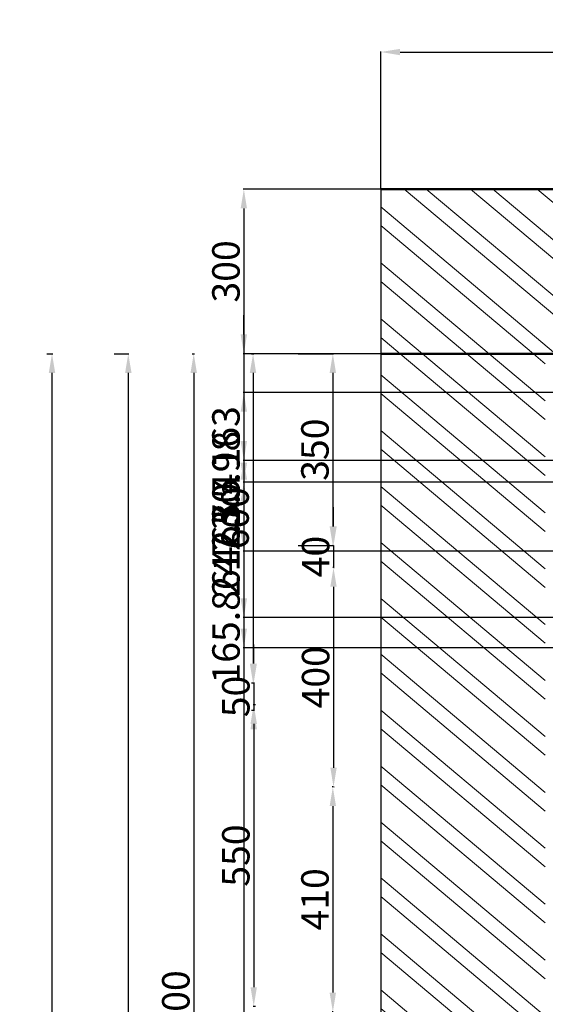
# Model space of a CAD drawing. Units: millimetres. Extents: x 407065 to 421840, y 1168257 to 1177792.
# Tile 5 of 17: x 407065 to 408024, y 1175951 to 1177747. Entities that reach past the tile are written whole.
import ezdxf

# ---------------------------------------------------------------- set-up
doc = ezdxf.new("R2010")
doc.units = ezdxf.units.MM
for name, color, linetype, lineweight in [('A-ANNO-DIMS', 6, 'Continuous', 18), ('A-FURN', 3, 'Continuous', 25), ('A-WALL', 7, 'Continuous', 50), ('A-WALL-PATT', 8, 'Continuous', 13)]:
    doc.layers.add(name, color=color, linetype=linetype, lineweight=lineweight)
doc.styles.get("Standard").update_dxf_attribs({"font": 'arial.ttf'})
doc.dimstyles.new('ISO-25', dxfattribs={"dimtxt": 50, "dimasz": 35, "dimexe": 1.25, "dimexo": 0.625, "dimtad": 1, "dimdec": 1, "dimtxsty": 'Standard', "dimcen": 35, "dimadec": 0, "dimazin": 0, "dimtfac": 1, "dimtdec": 1, "dimtmove": 0, "dimatfit": 3, "dimfxl": 1, "dimarcsym": 0})

# ---------------------------------------------------------------- blocks, each defined once
blk = doc.blocks.new('*D37')
at = {"layer": 'A-ANNO-DIMS', "color": 0, "lineweight": -2, "transparency": 16777216}
for p, q in [((407573.3, 1177137.8), (407637.9, 1177137.8)), ((407636.7, 1177102.8), (407636.7, 1176822.8)), ((407573.3, 1176787.8), (407637.9, 1176787.8))]:
    blk.add_line(p, q, dxfattribs=at)
at = {"layer": 'A-ANNO-DIMS', "color": 0, "transparency": 16777216}
for points in [[(407630.8, 1177102.8), (407642.5, 1177102.8), (407636.7, 1177137.8)], [(407630.8, 1176822.8), (407642.5, 1176822.8), (407636.7, 1176787.8)]]:
    blk.add_solid(points, dxfattribs=at)
at = {"layer": 'Defpoints', "color": 0, "transparency": 16777216}
for p in [(407572.7, 1177137.8), (407572.7, 1176787.8), (407636.7, 1176787.8)]:
    blk.add_point(p, dxfattribs=at)
at = {"layer": 'A-ANNO-DIMS', "color": 0, "transparency": 16777216, "insert": (407610.5, 1176962.8), "char_height": 50, "attachment_point": 5, "rotation": 90}
blk.add_mtext('350', dxfattribs=at)
blk = doc.blocks.new('*D38')
at = {"layer": 'A-ANNO-DIMS', "color": 0, "lineweight": -2, "transparency": 16777216}
for p, q in [((407637.9, 1176822.8), (407637.9, 1176857.8)), ((407637.3, 1176787.8), (407636.7, 1176787.8)), ((407637.9, 1176787.8), (407637.9, 1176747.8)), ((407637.3, 1176747.8), (407636.7, 1176747.8)), ((407637.9, 1176712.8), (407637.9, 1176677.8))]:
    blk.add_line(p, q, dxfattribs=at)
at = {"layer": 'A-ANNO-DIMS', "color": 0, "transparency": 16777216}
for points in [[(407632.1, 1176822.8), (407643.7, 1176822.8), (407637.9, 1176787.8)], [(407632.1, 1176712.8), (407643.7, 1176712.8), (407637.9, 1176747.8)]]:
    blk.add_solid(points, dxfattribs=at)
at = {"layer": 'Defpoints', "color": 0, "transparency": 16777216}
for p in [(407637.9, 1176787.8), (407637.9, 1176747.8), (407637.9, 1176747.8)]:
    blk.add_point(p, dxfattribs=at)
at = {"layer": 'A-ANNO-DIMS', "color": 0, "transparency": 16777216, "insert": (407611.7, 1176767.8), "char_height": 50, "attachment_point": 5, "rotation": 90}
blk.add_mtext('40', dxfattribs=at)
blk = doc.blocks.new('*D39')
at = {"layer": 'A-ANNO-DIMS', "color": 0, "lineweight": -2, "transparency": 16777216}
for p, q in [((407638.5, 1176747.8), (407639.2, 1176747.8)), ((407637.9, 1176712.8), (407637.9, 1176382.8)), ((407638.5, 1176347.8), (407639.2, 1176347.8))]:
    blk.add_line(p, q, dxfattribs=at)
at = {"layer": 'A-ANNO-DIMS', "color": 0, "transparency": 16777216}
for points in [[(407632.1, 1176712.8), (407643.7, 1176712.8), (407637.9, 1176747.8)], [(407632.1, 1176382.8), (407643.7, 1176382.8), (407637.9, 1176347.8)]]:
    blk.add_solid(points, dxfattribs=at)
at = {"layer": 'Defpoints', "color": 0, "transparency": 16777216}
for p in [(407637.9, 1176747.8), (407637.9, 1176347.8), (407637.9, 1176347.8)]:
    blk.add_point(p, dxfattribs=at)
at = {"layer": 'A-ANNO-DIMS', "color": 0, "transparency": 16777216, "insert": (407611.7, 1176547.8), "char_height": 50, "attachment_point": 5, "rotation": 90}
blk.add_mtext('400', dxfattribs=at)
blk = doc.blocks.new('*D40')
at = {"layer": 'A-ANNO-DIMS', "color": 0, "lineweight": -2, "transparency": 16777216}
for p, q in [((407637.3, 1176347.8), (407635.4, 1176347.8)), ((407636.7, 1176312.8), (407636.7, 1175972.8)), ((407637.3, 1175937.8), (407635.4, 1175937.8))]:
    blk.add_line(p, q, dxfattribs=at)
at = {"layer": 'A-ANNO-DIMS', "color": 0, "transparency": 16777216}
for points in [[(407630.8, 1176312.8), (407642.5, 1176312.8), (407636.7, 1176347.8)], [(407630.8, 1175972.8), (407642.5, 1175972.8), (407636.7, 1175937.8)]]:
    blk.add_solid(points, dxfattribs=at)
at = {"layer": 'Defpoints', "color": 0, "transparency": 16777216}
for p in [(407637.9, 1176347.8), (407636.7, 1175937.8), (407637.9, 1175937.8)]:
    blk.add_point(p, dxfattribs=at)
at = {"layer": 'A-ANNO-DIMS', "color": 0, "transparency": 16777216, "insert": (407610.5, 1176142.8), "char_height": 50, "attachment_point": 5, "rotation": 90}
blk.add_mtext('410', dxfattribs=at)
blk = doc.blocks.new('*D44')
at = {"layer": 'A-ANNO-DIMS', "color": 0, "lineweight": -2, "transparency": 16777216}
for p, q in [((407488.5, 1177137.8), (407492.3, 1177137.8)), ((407491.1, 1177102.8), (407491.1, 1176572.8)), ((407488.5, 1176537.8), (407492.3, 1176537.8))]:
    blk.add_line(p, q, dxfattribs=at)
at = {"layer": 'A-ANNO-DIMS', "color": 0, "transparency": 16777216}
for points in [[(407485.2, 1177102.8), (407496.9, 1177102.8), (407491.1, 1177137.8)], [(407485.2, 1176572.8), (407496.9, 1176572.8), (407491.1, 1176537.8)]]:
    blk.add_solid(points, dxfattribs=at)
at = {"layer": 'Defpoints', "color": 0, "transparency": 16777216}
for p in [(407487.8, 1177137.8), (407487.8, 1176537.8), (407491.1, 1176537.8)]:
    blk.add_point(p, dxfattribs=at)
at = {"layer": 'A-ANNO-DIMS', "color": 0, "transparency": 16777216, "insert": (407464.9, 1176837.8), "char_height": 50, "attachment_point": 5, "rotation": 90}
blk.add_mtext('600', dxfattribs=at)
blk = doc.blocks.new('*D45')
at = {"layer": 'A-ANNO-DIMS', "color": 0, "lineweight": -2, "transparency": 16777216}
for p, q in [((407492.3, 1176572.8), (407492.3, 1176607.8)), ((407488.5, 1176537.8), (407493.6, 1176537.8)), ((407492.3, 1176537.8), (407492.3, 1176487.8)), ((407488.5, 1176487.8), (407493.6, 1176487.8)), ((407492.3, 1176452.8), (407492.3, 1176417.8))]:
    blk.add_line(p, q, dxfattribs=at)
at = {"layer": 'A-ANNO-DIMS', "color": 0, "transparency": 16777216}
for points in [[(407486.5, 1176572.8), (407498.2, 1176572.8), (407492.3, 1176537.8)], [(407486.5, 1176452.8), (407498.2, 1176452.8), (407492.3, 1176487.8)]]:
    blk.add_solid(points, dxfattribs=at)
at = {"layer": 'Defpoints', "color": 0, "transparency": 16777216}
for p in [(407487.8, 1176537.8), (407487.8, 1176487.8), (407492.3, 1176487.8)]:
    blk.add_point(p, dxfattribs=at)
at = {"layer": 'A-ANNO-DIMS', "color": 0, "transparency": 16777216, "insert": (407466.2, 1176512.8), "char_height": 50, "attachment_point": 5, "rotation": 90}
blk.add_mtext('50', dxfattribs=at)
blk = doc.blocks.new('*D46')
at = {"layer": 'A-ANNO-DIMS', "color": 0, "lineweight": -2, "transparency": 16777216}
for p, q in [((407495.4, 1176497.7), (407491.1, 1176497.7)), ((407492.3, 1176462.7), (407492.3, 1175982.7)), ((407495.4, 1175947.7), (407491.1, 1175947.7))]:
    blk.add_line(p, q, dxfattribs=at)
at = {"layer": 'A-ANNO-DIMS', "color": 0, "transparency": 16777216}
for points in [[(407486.5, 1176462.7), (407498.2, 1176462.7), (407492.3, 1176497.7)], [(407486.5, 1175982.7), (407498.2, 1175982.7), (407492.3, 1175947.7)]]:
    blk.add_solid(points, dxfattribs=at)
at = {"layer": 'Defpoints', "color": 0, "transparency": 16777216}
for p in [(407496.1, 1176497.7), (407492.3, 1175947.7), (407496.1, 1175947.7)]:
    blk.add_point(p, dxfattribs=at)
at = {"layer": 'A-ANNO-DIMS', "color": 0, "transparency": 16777216, "insert": (407466.2, 1176222.7), "char_height": 50, "attachment_point": 5, "rotation": 90}
blk.add_mtext('550', dxfattribs=at)
blk = doc.blocks.new('*D49')
at = {"layer": 'A-ANNO-DIMS', "color": 0, "lineweight": -2, "transparency": 16777216}
for p, q in [((407380.2, 1177137.8), (407384.1, 1177137.8)), ((407382.9, 1177102.8), (407382.9, 1174772.8)), ((407380.2, 1174737.8), (407384.1, 1174737.8))]:
    blk.add_line(p, q, dxfattribs=at)
at = {"layer": 'A-ANNO-DIMS', "color": 0, "transparency": 16777216}
for points in [[(407377, 1177102.8), (407388.7, 1177102.8), (407382.9, 1177137.8)], [(407377, 1174772.8), (407388.7, 1174772.8), (407382.9, 1174737.8)]]:
    blk.add_solid(points, dxfattribs=at)
at = {"layer": 'Defpoints', "color": 0, "transparency": 16777216}
for p in [(407379.6, 1177137.8), (407379.6, 1174737.8), (407382.9, 1174737.8)]:
    blk.add_point(p, dxfattribs=at)
at = {"layer": 'A-ANNO-DIMS', "color": 0, "transparency": 16777216, "insert": (407356.7, 1175937.8), "char_height": 50, "attachment_point": 5, "rotation": 90}
blk.add_mtext('2400', dxfattribs=at)
blk = doc.blocks.new('*D50')
at = {"layer": 'A-ANNO-DIMS', "color": 0, "lineweight": -2, "transparency": 16777216}
for p, q in [((407237.7, 1177137.8), (407264.8, 1177137.8)), ((407263.5, 1177102.8), (407263.5, 1174502.8)), ((407237.7, 1174467.8), (407264.8, 1174467.8))]:
    blk.add_line(p, q, dxfattribs=at)
at = {"layer": 'A-ANNO-DIMS', "color": 0, "transparency": 16777216}
for points in [[(407257.7, 1177102.8), (407269.4, 1177102.8), (407263.5, 1177137.8)], [(407257.7, 1174502.8), (407269.4, 1174502.8), (407263.5, 1174467.8)]]:
    blk.add_solid(points, dxfattribs=at)
at = {"layer": 'Defpoints', "color": 0, "transparency": 16777216}
for p in [(407237, 1177137.8), (407237, 1174467.8), (407263.5, 1174467.8)]:
    blk.add_point(p, dxfattribs=at)
at = {"layer": 'A-ANNO-DIMS', "color": 0, "transparency": 16777216, "insert": (407237.4, 1175802.8), "char_height": 50, "attachment_point": 5, "rotation": 90}
blk.add_mtext('2670', dxfattribs=at)
blk = doc.blocks.new('*D51')
at = {"layer": 'A-ANNO-DIMS', "color": 0, "lineweight": -2, "transparency": 16777216}
for p, q in [((407115, 1177137.8), (407125.6, 1177137.8)), ((407124.3, 1177102.8), (407124.3, 1173382.8)), ((407115, 1173347.8), (407125.6, 1173347.8))]:
    blk.add_line(p, q, dxfattribs=at)
at = {"layer": 'A-ANNO-DIMS', "color": 0, "transparency": 16777216}
for points in [[(407118.5, 1177102.8), (407130.2, 1177102.8), (407124.3, 1177137.8)], [(407118.5, 1173382.8), (407130.2, 1173382.8), (407124.3, 1173347.8)]]:
    blk.add_solid(points, dxfattribs=at)
at = {"layer": 'Defpoints', "color": 0, "transparency": 16777216}
for p in [(407114.4, 1177137.8), (407114.4, 1173347.8), (407124.3, 1173347.8)]:
    blk.add_point(p, dxfattribs=at)
at = {"layer": 'A-ANNO-DIMS', "color": 0, "transparency": 16777216, "insert": (407098.2, 1175242.8), "char_height": 50, "attachment_point": 5, "rotation": 90}
blk.add_mtext('3790', dxfattribs=at)
blk = doc.blocks.new('*D165')
at = {"layer": 'A-ANNO-DIMS', "color": 0, "lineweight": -2, "transparency": 16777216}
for p, q in [((407724.3, 1177438.4), (407724.3, 1177689)), ((407759.3, 1177687.8), (410989.3, 1177687.8)), ((411024.3, 1177438.4), (411024.3, 1177689))]:
    blk.add_line(p, q, dxfattribs=at)
at = {"layer": 'A-ANNO-DIMS', "color": 0, "transparency": 16777216}
for points in [[(407759.3, 1177693.6), (407759.3, 1177682), (407724.3, 1177687.8)], [(410989.3, 1177693.6), (410989.3, 1177682), (411024.3, 1177687.8)]]:
    blk.add_solid(points, dxfattribs=at)
at = {"layer": 'Defpoints', "color": 0, "transparency": 16777216}
for p in [(411024.3, 1177687.8), (407724.3, 1177437.8), (411024.3, 1177437.8)]:
    blk.add_point(p, dxfattribs=at)
at = {"layer": 'A-ANNO-DIMS', "color": 0, "transparency": 16777216, "insert": (409374.3, 1177714), "char_height": 50, "attachment_point": 5}
blk.add_mtext('3300', dxfattribs=at)
blk = doc.blocks.new('*D166')
at = {"layer": 'A-ANNO-DIMS', "color": 0, "lineweight": -2, "transparency": 16777216}
for p, q in [((407723.7, 1177437.8), (407473.1, 1177437.8)), ((407474.3, 1177402.8), (407474.3, 1173182.8)), ((407723.7, 1173147.8), (407473.1, 1173147.8))]:
    blk.add_line(p, q, dxfattribs=at)
at = {"layer": 'A-ANNO-DIMS', "color": 0, "transparency": 16777216}
for points in [[(407468.5, 1177402.8), (407480.1, 1177402.8), (407474.3, 1177437.8)], [(407468.5, 1173182.8), (407480.1, 1173182.8), (407474.3, 1173147.8)]]:
    blk.add_solid(points, dxfattribs=at)
at = {"layer": 'Defpoints', "color": 0, "transparency": 16777216}
for p in [(407724.3, 1177437.8), (407474.3, 1173147.8), (407724.3, 1173147.8)]:
    blk.add_point(p, dxfattribs=at)
at = {"layer": 'A-ANNO-DIMS', "color": 0, "transparency": 16777216, "insert": (407448.2, 1175292.8), "char_height": 50, "attachment_point": 5, "rotation": 90}
blk.add_mtext('4290', dxfattribs=at)
blk = doc.blocks.new('*D168')
at = {"layer": 'A-ANNO-DIMS', "color": 0, "lineweight": -2, "transparency": 16777216}
for p, q in [((407723.7, 1177437.8), (407473.1, 1177437.8)), ((407474.3, 1177402.8), (407474.3, 1177172.8)), ((408023.7, 1177137.8), (407473.1, 1177137.8))]:
    blk.add_line(p, q, dxfattribs=at)
at = {"layer": 'A-ANNO-DIMS', "color": 0, "transparency": 16777216}
for points in [[(407468.5, 1177402.8), (407480.1, 1177402.8), (407474.3, 1177437.8)], [(407468.5, 1177172.8), (407480.1, 1177172.8), (407474.3, 1177137.8)]]:
    blk.add_solid(points, dxfattribs=at)
at = {"layer": 'Defpoints', "color": 0, "transparency": 16777216}
for p in [(407724.3, 1177437.8), (407474.3, 1177137.8), (408024.3, 1177137.8)]:
    blk.add_point(p, dxfattribs=at)
at = {"layer": 'A-ANNO-DIMS', "color": 0, "transparency": 16777216, "insert": (407448.1, 1177287.8), "char_height": 50, "attachment_point": 5, "rotation": 90}
blk.add_mtext('300', dxfattribs=at)
blk = doc.blocks.new('*D172')
at = {"layer": 'A-ANNO-DIMS', "color": 0, "lineweight": -2, "transparency": 16777216}
for p, q in [((408655, 1177066.8), (407473.1, 1177066.8)), ((407474.3, 1177031.8), (407474.3, 1176636.4)), ((408655, 1176601.4), (407473.1, 1176601.4))]:
    blk.add_line(p, q, dxfattribs=at)
at = {"layer": 'A-ANNO-DIMS', "color": 0, "transparency": 16777216}
for points in [[(407468.5, 1177031.8), (407480.1, 1177031.8), (407474.3, 1177066.8)], [(407468.5, 1176636.4), (407480.1, 1176636.4), (407474.3, 1176601.4)]]:
    blk.add_solid(points, dxfattribs=at)
at = {"layer": 'Defpoints', "color": 0, "transparency": 16777216}
for p in [(408655.7, 1177066.8), (407474.3, 1176601.4), (408655.7, 1176601.4)]:
    blk.add_point(p, dxfattribs=at)
at = {"layer": 'A-ANNO-DIMS', "color": 0, "transparency": 16777216, "insert": (407448.2, 1176834.1), "char_height": 50, "attachment_point": 5, "rotation": 90}
blk.add_mtext('465.4', dxfattribs=at)
blk = doc.blocks.new('*D173')
at = {"layer": 'A-ANNO-DIMS', "color": 0, "lineweight": -2, "transparency": 16777216}
for p, q in [((407474.3, 1177172.8), (407474.3, 1177207.8)), ((408573.7, 1177137.8), (407473.1, 1177137.8)), ((407474.3, 1177137.8), (407474.3, 1177066.8)), ((408655, 1177066.8), (407473.1, 1177066.8)), ((407474.3, 1177031.8), (407474.3, 1176827.1))]:
    blk.add_line(p, q, dxfattribs=at)
at = {"layer": 'A-ANNO-DIMS', "color": 0, "transparency": 16777216}
for points in [[(407468.5, 1177172.8), (407480.1, 1177172.8), (407474.3, 1177137.8)], [(407468.5, 1177031.8), (407480.1, 1177031.8), (407474.3, 1177066.8)]]:
    blk.add_solid(points, dxfattribs=at)
at = {"layer": 'Defpoints', "color": 0, "transparency": 16777216}
for p in [(408574.3, 1177137.8), (407474.3, 1177066.8), (408655.7, 1177066.8)]:
    blk.add_point(p, dxfattribs=at)
at = {"layer": 'A-ANNO-DIMS', "color": 0, "transparency": 16777216, "insert": (407448.2, 1176912), "char_height": 50, "attachment_point": 5, "rotation": 90}
blk.add_mtext('70.98', dxfattribs=at)
blk = doc.blocks.new('*D175')
at = {"layer": 'A-ANNO-DIMS', "color": 0, "lineweight": -2, "transparency": 16777216}
for p, q in [((408668.9, 1176903.8), (407473.1, 1176903.8)), ((407474.3, 1176868.8), (407474.3, 1176691.5)), ((408668.9, 1176656.5), (407473.1, 1176656.5))]:
    blk.add_line(p, q, dxfattribs=at)
at = {"layer": 'A-ANNO-DIMS', "color": 0, "transparency": 16777216}
for points in [[(407468.5, 1176868.8), (407480.1, 1176868.8), (407474.3, 1176903.8)], [(407468.5, 1176691.5), (407480.1, 1176691.5), (407474.3, 1176656.5)]]:
    blk.add_solid(points, dxfattribs=at)
at = {"layer": 'Defpoints', "color": 0, "transparency": 16777216}
for p in [(408669.5, 1176903.8), (407474.3, 1176656.5), (408669.5, 1176656.5)]:
    blk.add_point(p, dxfattribs=at)
at = {"layer": 'A-ANNO-DIMS', "color": 0, "transparency": 16777216, "insert": (407448.1, 1176780.2), "char_height": 50, "attachment_point": 5, "rotation": 90}
blk.add_mtext('247.3', dxfattribs=at)
blk = doc.blocks.new('*D177')
at = {"layer": 'A-ANNO-DIMS', "color": 0, "lineweight": -2, "transparency": 16777216}
for p, q in [((408655, 1177066.8), (407473.1, 1177066.8)), ((407474.3, 1177031.8), (407474.3, 1176938.8)), ((408668.9, 1176903.8), (407473.1, 1176903.8))]:
    blk.add_line(p, q, dxfattribs=at)
at = {"layer": 'A-ANNO-DIMS', "color": 0, "transparency": 16777216}
for points in [[(407468.5, 1177031.8), (407480.1, 1177031.8), (407474.3, 1177066.8)], [(407468.5, 1176938.8), (407480.1, 1176938.8), (407474.3, 1176903.8)]]:
    blk.add_solid(points, dxfattribs=at)
at = {"layer": 'Defpoints', "color": 0, "transparency": 16777216}
for p in [(408655.7, 1177066.8), (407474.3, 1176903.8), (408669.5, 1176903.8)]:
    blk.add_point(p, dxfattribs=at)
at = {"layer": 'A-ANNO-DIMS', "color": 0, "transparency": 16777216, "insert": (407448.1, 1176985.3), "char_height": 50, "attachment_point": 5, "rotation": 90}
blk.add_mtext('163', dxfattribs=at)
blk = doc.blocks.new('*D182')
at = {"layer": 'A-ANNO-DIMS', "color": 0, "lineweight": -2, "transparency": 16777216}
for p, q in [((409505, 1177066.8), (407473.1, 1177066.8)), ((407474.3, 1177031.8), (407474.3, 1176978.3)), ((409523.4, 1176943.3), (407473.1, 1176943.3)), ((407474.3, 1176943.3), (407474.3, 1176742.7))]:
    blk.add_line(p, q, dxfattribs=at)
at = {"layer": 'A-ANNO-DIMS', "color": 0, "transparency": 16777216}
for points in [[(407468.5, 1177031.8), (407480.1, 1177031.8), (407474.3, 1177066.8)], [(407468.5, 1176978.3), (407480.1, 1176978.3), (407474.3, 1176943.3)]]:
    blk.add_solid(points, dxfattribs=at)
at = {"layer": 'Defpoints', "color": 0, "transparency": 16777216}
for p in [(409505.7, 1177066.8), (407474.3, 1176943.3), (409524, 1176943.3)]:
    blk.add_point(p, dxfattribs=at)
at = {"layer": 'A-ANNO-DIMS', "color": 0, "transparency": 16777216, "insert": (407448.1, 1176825.5), "char_height": 50, "attachment_point": 5, "rotation": 90}
blk.add_mtext('123.5', dxfattribs=at)
blk = doc.blocks.new('*D183')
at = {"layer": 'A-ANNO-DIMS', "color": 0, "lineweight": -2, "transparency": 16777216}
for p, q in [((409523.4, 1176943.3), (407473.1, 1176943.3)), ((407474.3, 1176908.3), (407474.3, 1176812.5)), ((409523.4, 1176777.5), (407473.1, 1176777.5)), ((407474.3, 1176777.5), (407474.3, 1176538.4))]:
    blk.add_line(p, q, dxfattribs=at)
at = {"layer": 'A-ANNO-DIMS', "color": 0, "transparency": 16777216}
for points in [[(407468.5, 1176908.3), (407480.1, 1176908.3), (407474.3, 1176943.3)], [(407468.5, 1176812.5), (407480.1, 1176812.5), (407474.3, 1176777.5)]]:
    blk.add_solid(points, dxfattribs=at)
at = {"layer": 'Defpoints', "color": 0, "transparency": 16777216}
for p in [(409524, 1176943.3), (407474.3, 1176777.5), (409524, 1176777.5)]:
    blk.add_point(p, dxfattribs=at)
at = {"layer": 'A-ANNO-DIMS', "color": 0, "transparency": 16777216, "insert": (407448.2, 1176640.4), "char_height": 50, "attachment_point": 5, "rotation": 90}
blk.add_mtext('165.86', dxfattribs=at)

msp = doc.modelspace()

# ---------------------------------------------------------------- hatches: boundary and pattern name
at = {"layer": 'A-WALL-PATT'}
h = msp.add_hatch(dxfattribs=at)
h.set_pattern_fill('ANSI32', color=256, scale=8.2, angle=95)
h.paths.add_polyline_path([(411024.3133, 1177437.7952), (407724.3133, 1177437.7952), (407724.3133, 1177137.7952), (408024.3133, 1177137.7952), (410824.3133, 1177137.7952), (411024.3133, 1177137.7952)])
h = msp.add_hatch(dxfattribs=at)
h.set_pattern_fill('ANSI32', color=256, scale=8.2, angle=95)
h.paths.add_polyline_path([(408024.3133, 1177137.7952), (407724.3133, 1177137.7952), (407724.3133, 1174467.7952), (408024.3133, 1174467.7952)])

# ---------------------------------------------------------------- linework, layer by layer
at = {"layer": 'A-FURN'}
msp.add_line((407724.3133, 1177437.7952), (407724.3133, 1174467.7952), dxfattribs=at)
at = {"layer": 'A-WALL'}
for p, q in [((411024.3133, 1177437.7952), (407724.3133, 1177437.7952)), ((408024.3133, 1177137.7952), (407724.3133, 1177137.7952)), ((410824.3133, 1177137.7952), (408024.3133, 1177137.7952))]:
    msp.add_line(p, q, dxfattribs=at)

# ---------------------------------------------------------------- dimensions: what is measured, and where the dimension line sits
at = {"layer": 'A-ANNO-DIMS'}
dim = msp.add_linear_dim(base=(411024.3133, 1177687.7952), p1=(407724.3133, 1177437.7952), p2=(411024.3133, 1177437.7952), dimstyle='ISO-25', override={"dimdec": 0, "dimlfac": 1, "dimrnd": 0, "dimzin": 0, "dimdsep": 46, "dimlunit": 2}, dxfattribs=at)
dim.commit()
dim.dimension.update_dxf_attribs({"geometry": '*D165', "text_midpoint": (409374.3133, 1177713.9659)})
for base, p1, p2, override, picture, middle in [((407474.3133, 1177137.7952), (407724.3133, 1177437.7952), (408024.3133, 1177137.7952), {"dimdec": 0, "dimlfac": 1, "dimrnd": 0, "dimzin": 0, "dimdsep": 46, "dimlunit": 2}, '*D168', (407448.1426, 1177287.7952)), ((407474.3133, 1173147.7952), (407724.3133, 1177437.7952), (407724.3133, 1173147.7952), {"dimdec": 0, "dimlfac": 1, "dimrnd": 0, "dimzin": 0, "dimdsep": 46, "dimlunit": 2}, '*D166', (407448.1597, 1175292.7952)), ((407474.3133, 1177066.8168), (408574.3133, 1177137.7952), (408655.6554, 1177066.8168), {"dimdec": 2, "dimlfac": 1, "dimrnd": 0, "dimzin": 0, "dimdsep": 46, "dimlunit": 2}, '*D173', (407448.1597, 1176911.983)), ((407124.3456, 1173347.7952), (407114.4021, 1177137.7952), (407114.4021, 1173347.7952), {"dimclrd": 0, "dimclre": 0, "dimclrt": 0}, '*D51', (407098.1749, 1175242.7952)), ((407263.5498, 1174467.7952), (407237.0345, 1177137.7952), (407237.0345, 1174467.7952), {"dimclrd": 0, "dimclre": 0, "dimclrt": 0}, '*D50', (407237.3961, 1175802.7952)), ((407382.8674, 1174737.7952), (407379.577, 1177137.7952), (407379.577, 1174737.7952), {"dimclrd": 0, "dimclre": 0, "dimclrt": 0}, '*D49', (407356.7137, 1175937.7952)), ((407491.0711, 1176537.7952), (407487.8496, 1177137.7952), (407487.8496, 1176537.7952), {"dimclrd": 0, "dimclre": 0, "dimclrt": 0}, '*D44', (407464.9175, 1176837.7952)), ((407636.652, 1176787.7952), (407572.6583, 1177137.7952), (407572.6583, 1176787.7952), {"dimclrd": 0, "dimclre": 0, "dimclrt": 0}, '*D37', (407610.4813, 1176962.7952)), ((407474.3133, 1176903.8236), (408655.6554, 1177066.8168), (408669.5202, 1176903.8236), {"dimdec": 0, "dimlfac": 1, "dimrnd": 0, "dimzin": 0, "dimdsep": 46, "dimlunit": 2}, '*D177', (407448.1426, 1176985.3202)), ((407474.3133, 1176943.3161), (409505.6554, 1177066.8168), (409524.0157, 1176943.3161), {"dimdec": 1, "dimlfac": 1, "dimrnd": 0, "dimzin": 0, "dimdsep": 46, "dimlunit": 2}, '*D182', (407448.1426, 1176825.4947)), ((407474.3133, 1176601.4062), (408655.6554, 1177066.8168), (408655.6554, 1176601.4062), {"dimdec": 1, "dimlfac": 1, "dimrnd": 0, "dimzin": 0, "dimdsep": 46, "dimlunit": 2}, '*D172', (407448.1597, 1176834.1115)), ((407474.3133, 1176777.4536), (409524.0157, 1176943.3161), (409524.0157, 1176777.4536), {"dimdec": 2, "dimlfac": 1, "dimrnd": 0, "dimzin": 0, "dimdsep": 46, "dimlunit": 2}, '*D183', (407448.1597, 1176640.4132)), ((407474.3133, 1176656.5082), (408669.5202, 1176903.8236), (408669.5202, 1176656.5082), {"dimdec": 1, "dimlfac": 1, "dimrnd": 0, "dimzin": 0, "dimdsep": 46, "dimlunit": 2}, '*D175', (407448.1426, 1176780.1659)), ((407637.902, 1176347.7952), (407637.902, 1176747.7952), (407637.902, 1176347.7952), {"dimclrd": 0, "dimclre": 0, "dimclrt": 0}, '*D39', (407611.7483, 1176547.7952)), ((407492.3211, 1175947.6795), (407496.0711, 1176497.6795), (407496.0711, 1175947.6795), {"dimclrd": 0, "dimclre": 0, "dimclrt": 0}, '*D46', (407466.1675, 1176222.6795)), ((407636.652, 1175937.7952), (407637.902, 1176347.7952), (407637.902, 1175937.7952), {"dimclrd": 0, "dimclre": 0, "dimclrt": 0}, '*D40', (407610.4983, 1176142.7952))]:
    dim = msp.add_linear_dim(base=base, p1=p1, p2=p2, angle=90, dimstyle='ISO-25', override=override, dxfattribs=at)
    dim.commit()
    dim.dimension.update_dxf_attribs({"geometry": picture, "text_midpoint": middle})
for base, p1, p2, picture, middle in [((407637.902, 1176747.7952), (407637.902, 1176787.7952), (407637.902, 1176747.7952), '*D38', (407637.902, 1176767.7952)), ((407492.3211, 1176487.7952), (407487.8496, 1176537.7952), (407487.8496, 1176487.7952), '*D45', (407492.3211, 1176512.7952))]:
    dim = msp.add_linear_dim(base=base, p1=p1, p2=p2, angle=90, dimstyle='ISO-25', override={"dimclrd": 0, "dimclre": 0, "dimclrt": 0}, dxfattribs=at)
    dim.commit()
    dim.dimension.update_dxf_attribs({"geometry": picture, "text_midpoint": middle, "dimtype": 160})

doc.saveas('drawing.dxf')
